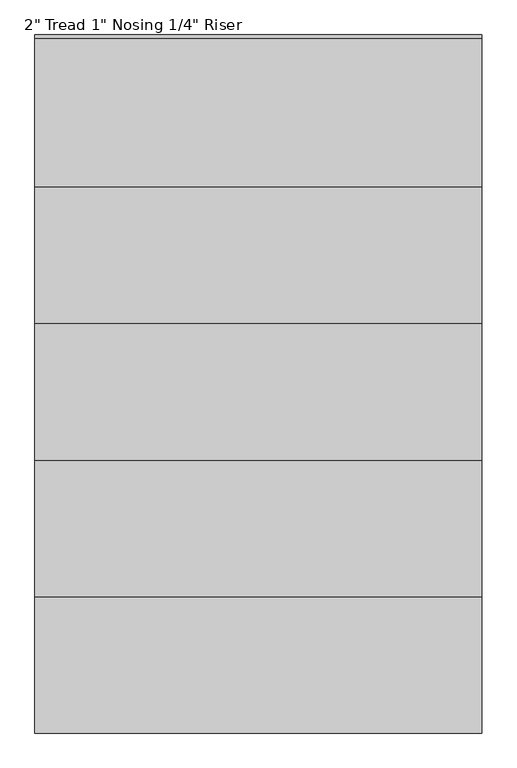
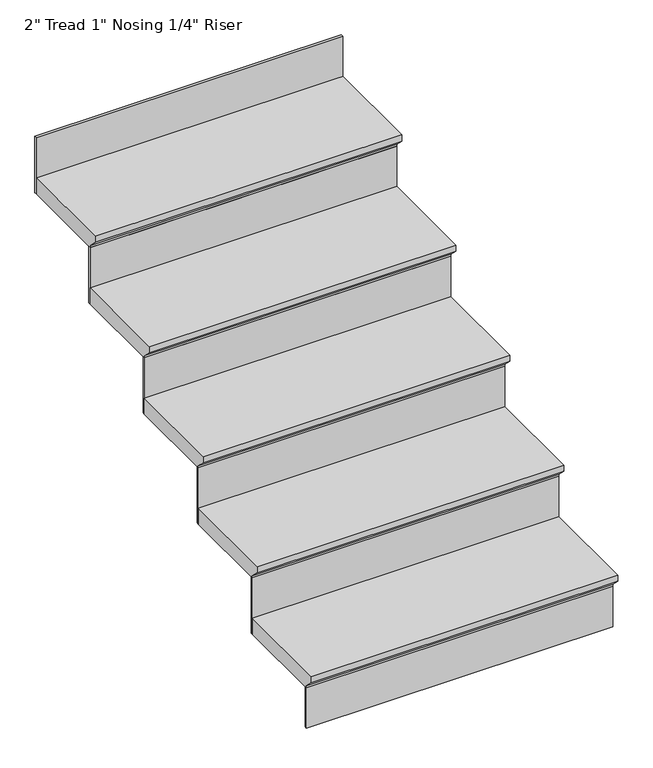
"""IFC4 building model written with IfcOpenShell, lengths in millimetres: stair flight geometry."""

from ifc_helpers import new_model, si_unit, frame, origin, place, context, project, spatial, polyline, outline, extrude, source, transform, mapped, element, save


def stair_flight_369be8b3(model_context):
    return source(origin(), model_context, "Body", "SweptSolid", [
        extrude(outline(polyline([(-2893.1217987, -889.0), (-2588.3217987, -889.0), (-2588.3217987, -939.8), (-2867.7217987, -939.8), (-2867.7217987, -933.45), (-2893.1217987, -908.05), (-2893.1217987, -889.0)])), frame((-3810.558803, 0.0, 0.0), z_axis=(1.0, 0.0, 0.0), x_axis=(0.0, 1.0, 0.0)), (0.0, 0.0, 1.0), 914.4),
        extrude(outline(polyline([(-2896.158803, -2861.3717987), (-2896.158803, -2867.7217987), (-3810.558803, -2867.7217987), (-3810.558803, -2861.3717987), (-2896.158803, -2861.3717987)])), frame((0.0, 0.0, -1066.8), z_axis=(0.0, 0.0, 1.0), x_axis=(1.0, 0.0, 0.0)), (0.0, 0.0, 1.0), 127.0),
        extrude(outline(polyline([(-2896.158803, -2581.9717987), (-2896.158803, -2588.3217987), (-3810.558803, -2588.3217987), (-3810.558803, -2581.9717987), (-2896.158803, -2581.9717987)])), frame((0.0, 0.0, -939.8), z_axis=(0.0, 0.0, 1.0), x_axis=(1.0, 0.0, 0.0)), (0.0, 0.0, 1.0), 177.8),
        extrude(outline(polyline([(-2613.7217987, -711.2), (-2308.9217987, -711.2), (-2308.9217987, -762.0), (-2588.3217987, -762.0), (-2588.3217987, -755.65), (-2613.7217987, -730.25), (-2613.7217987, -711.2)])), frame((-3810.558803, 0.0, 0.0), z_axis=(1.0, 0.0, 0.0), x_axis=(0.0, 1.0, 0.0)), (0.0, 0.0, 1.0), 914.4),
        extrude(outline(polyline([(-2896.158803, -2302.5717987), (-2896.158803, -2308.9217987), (-3810.558803, -2308.9217987), (-3810.558803, -2302.5717987), (-2896.158803, -2302.5717987)])), frame((0.0, 0.0, -762.0), z_axis=(0.0, 0.0, 1.0), x_axis=(1.0, 0.0, 0.0)), (0.0, 0.0, 1.0), 177.8),
        extrude(outline(polyline([(-2334.3217987, -533.4), (-2029.5217987, -533.4), (-2029.5217987, -584.2), (-2308.9217987, -584.2), (-2308.9217987, -577.85), (-2334.3217987, -552.45), (-2334.3217987, -533.4)])), frame((-3810.558803, 0.0, 0.0), z_axis=(1.0, 0.0, 0.0), x_axis=(0.0, 1.0, 0.0)), (0.0, 0.0, 1.0), 914.4),
        extrude(outline(polyline([(-2896.158803, -2023.1717987), (-2896.158803, -2029.5217987), (-3810.558803, -2029.5217987), (-3810.558803, -2023.1717987), (-2896.158803, -2023.1717987)])), frame((0.0, 0.0, -584.2), z_axis=(0.0, 0.0, 1.0), x_axis=(1.0, 0.0, 0.0)), (0.0, 0.0, 1.0), 177.8),
        extrude(outline(polyline([(-2054.9217987, -355.6), (-1750.1217987, -355.6), (-1750.1217987, -406.4), (-2029.5217987, -406.4), (-2029.5217987, -400.05), (-2054.9217987, -374.65), (-2054.9217987, -355.6)])), frame((-3810.558803, 0.0, 0.0), z_axis=(1.0, 0.0, 0.0), x_axis=(0.0, 1.0, 0.0)), (0.0, 0.0, 1.0), 914.4),
        extrude(outline(polyline([(-2896.158803, -1743.7717987), (-2896.158803, -1750.1217987), (-3810.558803, -1750.1217987), (-3810.558803, -1743.7717987), (-2896.158803, -1743.7717987)])), frame((0.0, 0.0, -406.4), z_axis=(0.0, 0.0, 1.0), x_axis=(1.0, 0.0, 0.0)), (0.0, 0.0, 1.0), 177.8),
        extrude(outline(polyline([(-2896.158803, -1464.3717987), (-2896.158803, -1470.7217987), (-3810.558803, -1470.7217987), (-3810.558803, -1464.3717987), (-2896.158803, -1464.3717987)])), frame((0.0, 0.0, -228.6), z_axis=(0.0, 0.0, 1.0), x_axis=(1.0, 0.0, 0.0)), (0.0, 0.0, 1.0), 177.8),
        extrude(outline(polyline([(-1775.5217987, -177.8), (-1470.7217987, -177.8), (-1470.7217987, -228.6), (-1750.1217987, -228.6), (-1750.1217987, -222.25), (-1775.5217987, -196.85), (-1775.5217987, -177.8)])), frame((-3810.558803, 0.0, 0.0), z_axis=(1.0, 0.0, 0.0), x_axis=(0.0, 1.0, 0.0)), (0.0, 0.0, 1.0), 914.4),
    ])


if __name__ == "__main__":
    model = new_model("IFC4")
    model_context = context("Model", 3, world=origin())
    ifc_project = project(units=[si_unit("LENGTHUNIT", "METRE", prefix="MILLI")], contexts=[model_context])
    site = spatial("IfcSite", under=ifc_project)
    building = spatial("IfcBuilding", under=site)
    placement = place(None, origin())
    stair_flight_shape = stair_flight_369be8b3(model_context)
    element("IfcStairFlight", 1, ObjectType="2\" Tread 1\" Nosing 1/4\" Riser", at=placement, inside=building, context=model_context, shape_type="MappedRepresentation", body=[
        mapped(stair_flight_shape, transform((0.0, 0.0, 0.0), x_axis=(1.0, 0.0, 0.0), y_axis=(0.0, 1.0, 0.0), z_axis=(0.0, 0.0, 1.0))),
    ])
    save(model, "model.ifc")
